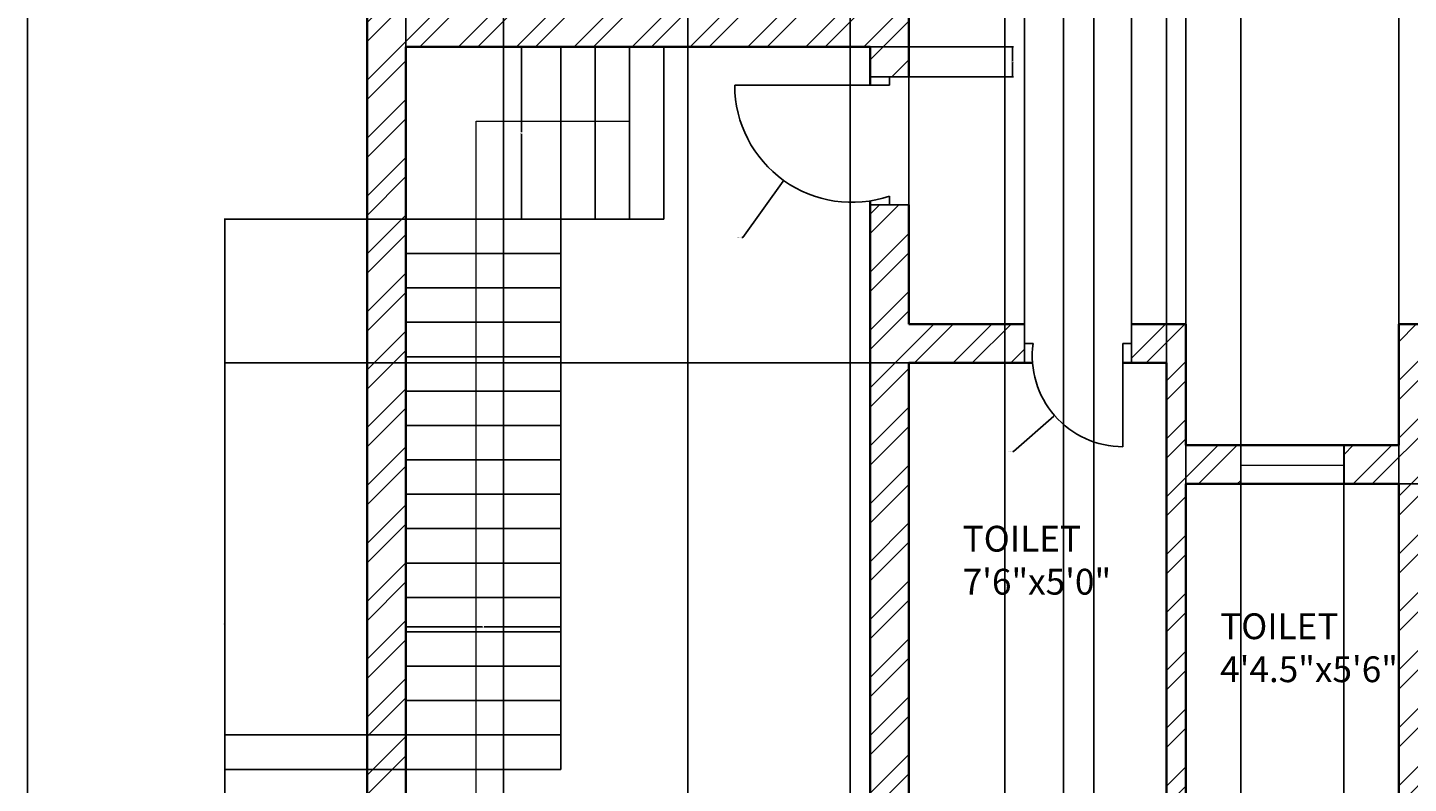
# Model space of a CAD drawing. Units: inches. Extents: x 1595 to 2135, y 460 to 2061.
# Tile 2 of 5: x 1595 to 1917, y 1470 to 1646. Entities that reach past the tile are written whole.
import ezdxf

# ---------------------------------------------------------------- set-up
doc = ezdxf.new("R2010")
doc.units = ezdxf.units.IN
for name, color, linetype, lineweight in [('A-ANNO-DIMS', 2, 'Continuous', 18), ('A-ANNO-SYMB', 7, 'Continuous', 18), ('A-ANNO-TTLB', 7, 'Continuous', 25), ('A-AREA-IDEN', 7, 'Continuous', 18), ('A-DOOR', 3, 'Continuous', 25), ('A-FLOR-STRS', 7, 'Continuous', 25), ('A-GLAZ', 4, 'Continuous', 18), ('A-WALL', 7, 'Continuous', 35)]:
    doc.layers.add(name, color=color, linetype=linetype, lineweight=lineweight)
doc.layers.add('A-WALL-PATT', color=143, linetype='Continuous', lineweight=13, true_color=0x7aafdf)
doc.styles.get("Standard").update_dxf_attribs({"font": 'arial.ttf'})
doc.dimstyles.get("Standard").update_dxf_attribs({"dimtxt": 0.18, "dimasz": 0.18, "dimexe": 0.18, "dimexo": 0.0625, "dimgap": 0.09, "dimtad": 0, "dimtih": 1, "dimtoh": 1, "dimdec": 4, "dimzin": 0, "dimdsep": 46, "dimtxsty": 'Standard', "dimcen": 0.09, "dimadec": 0, "dimazin": 0, "dimtfac": 1, "dimtdec": 4, "dimtofl": 0, "dimtmove": 0, "dimatfit": 3, "dimfxl": 1, "dimtolj": 1, "dimtzin": 0, "dimarcsym": 0})

# ---------------------------------------------------------------- blocks, each defined once
blk = doc.blocks.new('*D6')
at = {"layer": 'A-ANNO-DIMS', "color": 0, "lineweight": -2, "transparency": 16777216}
for p, q in [((1791.38, 1641.64), (1824.64, 1641.64)), ((1824.46, 1641.46), (1824.46, 1638.36)), ((1824.46, 1634.9), (1824.46, 1638)), ((1791.38, 1634.72), (1824.64, 1634.72))]:
    blk.add_line(p, q, dxfattribs=at)
at = {"layer": 'A-ANNO-DIMS', "color": 0, "transparency": 16777216}
for points in [[(1824.43, 1641.46), (1824.49, 1641.46), (1824.46, 1641.64)], [(1824.43, 1634.9), (1824.49, 1634.9), (1824.46, 1634.72)]]:
    blk.add_solid(points, dxfattribs=at)
at = {"layer": 'Defpoints', "color": 0, "transparency": 16777216}
for p in [(1791.31, 1641.64), (1791.31, 1634.72), (1824.46, 1634.72)]:
    blk.add_point(p, dxfattribs=at)
at = {"layer": 'A-ANNO-DIMS', "color": 0, "transparency": 16777216, "insert": (1824.46, 1638.18), "char_height": 0.18, "attachment_point": 5}
blk.add_mtext('\\A1;6.925', dxfattribs=at)
blk = doc.blocks.new('*D17')
at = {"layer": 'A-ANNO-DIMS', "color": 0, "lineweight": -2, "transparency": 16777216}
for p, q in [((1683.31, 1473.65), (1683.31, 1506.92)), ((1719.31, 1473.65), (1719.31, 1506.92)), ((1683.49, 1506.74), (1701.09, 1506.74)), ((1719.13, 1506.74), (1701.53, 1506.74))]:
    blk.add_line(p, q, dxfattribs=at)
at = {"layer": 'A-ANNO-DIMS', "color": 0, "transparency": 16777216}
for points in [[(1683.49, 1506.77), (1683.49, 1506.71), (1683.31, 1506.74)], [(1719.13, 1506.77), (1719.13, 1506.71), (1719.31, 1506.74)]]:
    blk.add_solid(points, dxfattribs=at)
at = {"layer": 'Defpoints', "color": 0, "transparency": 16777216}
for p in [(1719.31, 1506.74), (1683.31, 1473.59), (1719.31, 1473.59)]:
    blk.add_point(p, dxfattribs=at)
at = {"layer": 'A-ANNO-DIMS', "color": 0, "transparency": 16777216, "insert": (1701.31, 1506.74), "char_height": 0.18, "attachment_point": 5}
blk.add_mtext('\\A1;36', dxfattribs=at)
blk = doc.blocks.new('*D18')
at = {"layer": 'A-ANNO-DIMS', "color": 0, "lineweight": -2, "transparency": 16777216}
for p, q in [((1683.25, 1601.59), (1640.98, 1601.59)), ((1641.16, 1601.41), (1641.16, 1537.77)), ((1641.16, 1473.77), (1641.16, 1537.41)), ((1683.25, 1473.59), (1640.98, 1473.59))]:
    blk.add_line(p, q, dxfattribs=at)
at = {"layer": 'A-ANNO-DIMS', "color": 0, "transparency": 16777216}
for points in [[(1641.13, 1601.41), (1641.19, 1601.41), (1641.16, 1601.59)], [(1641.13, 1473.77), (1641.19, 1473.77), (1641.16, 1473.59)]]:
    blk.add_solid(points, dxfattribs=at)
at = {"layer": 'Defpoints', "color": 0, "transparency": 16777216}
for p in [(1641.16, 1601.59), (1683.31, 1601.59), (1683.31, 1473.59)]:
    blk.add_point(p, dxfattribs=at)
at = {"layer": 'A-ANNO-DIMS', "color": 0, "transparency": 16777216, "insert": (1641.16, 1537.59), "char_height": 0.18, "attachment_point": 5}
blk.add_mtext('\\A1;128', dxfattribs=at)
blk = doc.blocks.new('*D19')
at = {"layer": 'A-ANNO-DIMS', "color": 0, "lineweight": -2, "transparency": 16777216}
for p, q in [((1683.25, 1481.59), (1640.98, 1481.59)), ((1641.16, 1481.41), (1641.16, 1477.77)), ((1641.16, 1473.77), (1641.16, 1477.41)), ((1683.25, 1473.59), (1640.98, 1473.59))]:
    blk.add_line(p, q, dxfattribs=at)
at = {"layer": 'A-ANNO-DIMS', "color": 0, "transparency": 16777216}
for points in [[(1641.13, 1481.41), (1641.19, 1481.41), (1641.16, 1481.59)], [(1641.13, 1473.77), (1641.19, 1473.77), (1641.16, 1473.59)]]:
    blk.add_solid(points, dxfattribs=at)
at = {"layer": 'Defpoints', "color": 0, "transparency": 16777216}
for p in [(1641.16, 1481.59), (1683.31, 1481.59), (1683.31, 1473.59)]:
    blk.add_point(p, dxfattribs=at)
at = {"layer": 'A-ANNO-DIMS', "color": 0, "transparency": 16777216, "insert": (1641.16, 1477.59), "char_height": 0.18, "attachment_point": 5}
blk.add_mtext('\\A1;8', dxfattribs=at)
blk = doc.blocks.new('*D23')
at = {"layer": 'A-ANNO-DIMS', "color": 0, "lineweight": -2, "transparency": 16777216}
for p, q in [((1683.31, 1938.58), (1683.31, 1365.31)), ((1705.98, 1938.58), (1705.98, 1365.31)), ((1683.49, 1365.49), (1694.18, 1365.49)), ((1705.8, 1365.49), (1695.11, 1365.49))]:
    blk.add_line(p, q, dxfattribs=at)
at = {"layer": 'A-ANNO-DIMS', "color": 0, "transparency": 16777216}
for points in [[(1683.49, 1365.52), (1683.49, 1365.46), (1683.31, 1365.49)], [(1705.8, 1365.52), (1705.8, 1365.46), (1705.98, 1365.49)]]:
    blk.add_solid(points, dxfattribs=at)
at = {"layer": 'Defpoints', "color": 0, "transparency": 16777216}
for p in [(1683.31, 1938.64), (1705.98, 1938.64), (1705.98, 1365.49)]:
    blk.add_point(p, dxfattribs=at)
at = {"layer": 'A-ANNO-DIMS', "color": 0, "transparency": 16777216, "insert": (1694.64, 1365.49), "char_height": 0.18, "attachment_point": 5}
blk.add_mtext('\\A1;22.663', dxfattribs=at)
blk = doc.blocks.new('*D24')
at = {"layer": 'A-ANNO-DIMS', "color": 0, "lineweight": -2, "transparency": 16777216}
for p, q in [((1705.98, 1938.58), (1705.98, 1365.31)), ((1748.87, 1938.58), (1748.87, 1365.31)), ((1706.16, 1365.49), (1726.96, 1365.49)), ((1748.69, 1365.49), (1727.89, 1365.49))]:
    blk.add_line(p, q, dxfattribs=at)
at = {"layer": 'A-ANNO-DIMS', "color": 0, "transparency": 16777216}
for points in [[(1706.16, 1365.52), (1706.16, 1365.46), (1705.98, 1365.49)], [(1748.69, 1365.52), (1748.69, 1365.46), (1748.87, 1365.49)]]:
    blk.add_solid(points, dxfattribs=at)
at = {"layer": 'Defpoints', "color": 0, "transparency": 16777216}
for p in [(1705.98, 1938.64), (1748.87, 1938.64), (1748.87, 1365.49)]:
    blk.add_point(p, dxfattribs=at)
at = {"layer": 'A-ANNO-DIMS', "color": 0, "transparency": 16777216, "insert": (1727.42, 1365.49), "char_height": 0.18, "attachment_point": 5}
blk.add_mtext('\\A1;42.894', dxfattribs=at)
blk = doc.blocks.new('*D25')
at = {"layer": 'A-ANNO-DIMS', "color": 0, "lineweight": -2, "transparency": 16777216}
for p, q in [((1748.87, 1938.58), (1748.87, 1365.31)), ((1786.65, 1938.58), (1786.65, 1365.31)), ((1749.05, 1365.49), (1767.37, 1365.49)), ((1786.47, 1365.49), (1768.16, 1365.49))]:
    blk.add_line(p, q, dxfattribs=at)
at = {"layer": 'A-ANNO-DIMS', "color": 0, "transparency": 16777216}
for points in [[(1749.05, 1365.52), (1749.05, 1365.46), (1748.87, 1365.49)], [(1786.47, 1365.52), (1786.47, 1365.46), (1786.65, 1365.49)]]:
    blk.add_solid(points, dxfattribs=at)
at = {"layer": 'Defpoints', "color": 0, "transparency": 16777216}
for p in [(1748.87, 1938.64), (1786.65, 1938.64), (1786.65, 1365.49)]:
    blk.add_point(p, dxfattribs=at)
at = {"layer": 'A-ANNO-DIMS', "color": 0, "transparency": 16777216, "insert": (1767.76, 1365.49), "char_height": 0.18, "attachment_point": 5}
blk.add_mtext('\\A1;37.78', dxfattribs=at)
blk = doc.blocks.new('*D26')
at = {"layer": 'A-ANNO-DIMS', "color": 0, "lineweight": -2, "transparency": 16777216}
for p, q in [((1786.65, 1938.58), (1786.65, 1365.31)), ((1822.65, 1938.58), (1822.65, 1365.31)), ((1786.83, 1365.49), (1804.43, 1365.49)), ((1822.47, 1365.49), (1804.87, 1365.49))]:
    blk.add_line(p, q, dxfattribs=at)
at = {"layer": 'A-ANNO-DIMS', "color": 0, "transparency": 16777216}
for points in [[(1786.83, 1365.52), (1786.83, 1365.46), (1786.65, 1365.49)], [(1822.47, 1365.52), (1822.47, 1365.46), (1822.65, 1365.49)]]:
    blk.add_solid(points, dxfattribs=at)
at = {"layer": 'Defpoints', "color": 0, "transparency": 16777216}
for p in [(1786.65, 1938.64), (1822.65, 1938.64), (1822.65, 1365.49)]:
    blk.add_point(p, dxfattribs=at)
at = {"layer": 'A-ANNO-DIMS', "color": 0, "transparency": 16777216, "insert": (1804.65, 1365.49), "char_height": 0.18, "attachment_point": 5}
blk.add_mtext('\\A1;36', dxfattribs=at)
blk = doc.blocks.new('*D30')
at = {"layer": 'A-ANNO-DIMS', "color": 0, "lineweight": -2, "transparency": 16777216}
for p, q in [((1836.31, 1938.58), (1836.31, 1365.31)), ((1843.37, 1938.58), (1843.37, 1365.31)), ((1836.49, 1365.49), (1839.45, 1365.49)), ((1843.19, 1365.49), (1840.23, 1365.49))]:
    blk.add_line(p, q, dxfattribs=at)
at = {"layer": 'A-ANNO-DIMS', "color": 0, "transparency": 16777216}
for points in [[(1836.49, 1365.52), (1836.49, 1365.46), (1836.31, 1365.49)], [(1843.19, 1365.52), (1843.19, 1365.46), (1843.37, 1365.49)]]:
    blk.add_solid(points, dxfattribs=at)
at = {"layer": 'Defpoints', "color": 0, "transparency": 16777216}
for p in [(1836.31, 1938.64), (1843.37, 1938.64), (1843.37, 1365.49)]:
    blk.add_point(p, dxfattribs=at)
at = {"layer": 'A-ANNO-DIMS', "color": 0, "transparency": 16777216, "insert": (1839.84, 1365.49), "char_height": 0.18, "attachment_point": 5}
blk.add_mtext('\\A1;7.054', dxfattribs=at)
blk = doc.blocks.new('*D33')
at = {"layer": 'A-ANNO-DIMS', "color": 0, "lineweight": -2, "transparency": 16777216}
for p, q in [((1800.25, 1568.14), (1640.98, 1568.14)), ((1641.16, 1567.96), (1641.16, 1507.57)), ((1641.16, 1446.82), (1641.16, 1507.21)), ((1800.25, 1446.64), (1640.98, 1446.64))]:
    blk.add_line(p, q, dxfattribs=at)
at = {"layer": 'A-ANNO-DIMS', "color": 0, "transparency": 16777216}
for points in [[(1641.13, 1567.96), (1641.19, 1567.96), (1641.16, 1568.14)], [(1641.13, 1446.82), (1641.19, 1446.82), (1641.16, 1446.64)]]:
    blk.add_solid(points, dxfattribs=at)
at = {"layer": 'Defpoints', "color": 0, "transparency": 16777216}
for p in [(1641.16, 1568.14), (1800.31, 1568.14), (1800.31, 1446.64)]:
    blk.add_point(p, dxfattribs=at)
at = {"layer": 'A-ANNO-DIMS', "color": 0, "transparency": 16777216, "insert": (1641.16, 1507.39), "char_height": 0.18, "attachment_point": 5}
blk.add_mtext('\\A1;121.5', dxfattribs=at)
blk = doc.blocks.new('*D34')
at = {"layer": 'A-ANNO-DIMS', "color": 0, "lineweight": -2, "transparency": 16777216}
for p, q in [((1914.38, 1539.98), (2109.64, 1539.98)), ((2109.46, 1539.8), (2109.46, 1493.49)), ((2109.46, 1446.82), (2109.46, 1493.13)), ((1914.38, 1446.64), (2109.64, 1446.64))]:
    blk.add_line(p, q, dxfattribs=at)
at = {"layer": 'A-ANNO-DIMS', "color": 0, "transparency": 16777216}
for points in [[(2109.43, 1539.8), (2109.49, 1539.8), (2109.46, 1539.98)], [(2109.43, 1446.82), (2109.49, 1446.82), (2109.46, 1446.64)]]:
    blk.add_solid(points, dxfattribs=at)
at = {"layer": 'Defpoints', "color": 0, "transparency": 16777216}
for p in [(1914.31, 1539.98), (2109.46, 1539.98), (1914.31, 1446.64)]:
    blk.add_point(p, dxfattribs=at)
at = {"layer": 'A-ANNO-DIMS', "color": 0, "transparency": 16777216, "insert": (2109.46, 1493.31), "char_height": 0.18, "attachment_point": 5}
blk.add_mtext('\\A1;93.33', dxfattribs=at)
blk = doc.blocks.new('*D35')
at = {"layer": 'A-ANNO-DIMS', "color": 0, "lineweight": -2, "transparency": 16777216}
for p, q in [((1864.81, 1540.04), (1864.81, 2049.97)), ((1914.31, 1540.04), (1914.31, 2049.97)), ((1864.99, 2049.79), (1889.23, 2049.79)), ((1914.13, 2049.79), (1889.89, 2049.79))]:
    blk.add_line(p, q, dxfattribs=at)
at = {"layer": 'A-ANNO-DIMS', "color": 0, "transparency": 16777216}
for points in [[(1864.99, 2049.82), (1864.99, 2049.76), (1864.81, 2049.79)], [(1914.13, 2049.82), (1914.13, 2049.76), (1914.31, 2049.79)]]:
    blk.add_solid(points, dxfattribs=at)
at = {"layer": 'Defpoints', "color": 0, "transparency": 16777216}
for p in [(1914.31, 2049.79), (1864.81, 1539.98), (1914.31, 1539.98)]:
    blk.add_point(p, dxfattribs=at)
at = {"layer": 'A-ANNO-DIMS', "color": 0, "transparency": 16777216, "insert": (1889.56, 2049.79), "char_height": 0.18, "attachment_point": 5}
blk.add_mtext('\\A1;49.5', dxfattribs=at)
blk = doc.blocks.new('*D36')
at = {"layer": 'A-ANNO-DIMS', "color": 0, "lineweight": -2, "transparency": 16777216}
for p, q in [((1860.31, 1568.2), (1860.31, 2049.97)), ((1864.81, 1577.2), (1864.81, 2049.97)), ((1860.49, 2049.79), (1862.3, 2049.79)), ((1864.63, 2049.79), (1862.82, 2049.79))]:
    blk.add_line(p, q, dxfattribs=at)
at = {"layer": 'A-ANNO-DIMS', "color": 0, "transparency": 16777216}
for points in [[(1860.49, 2049.82), (1860.49, 2049.76), (1860.31, 2049.79)], [(1864.63, 2049.82), (1864.63, 2049.76), (1864.81, 2049.79)]]:
    blk.add_solid(points, dxfattribs=at)
at = {"layer": 'Defpoints', "color": 0, "transparency": 16777216}
for p in [(1864.81, 2049.79), (1864.81, 1577.14), (1860.31, 1568.14)]:
    blk.add_point(p, dxfattribs=at)
at = {"layer": 'A-ANNO-DIMS', "color": 0, "transparency": 16777216, "insert": (1862.56, 2049.79), "char_height": 0.18, "attachment_point": 5}
blk.add_mtext('\\A1;4.5', dxfattribs=at)
blk = doc.blocks.new('*D37')
at = {"layer": 'A-ANNO-DIMS', "color": 0, "lineweight": -2, "transparency": 16777216}
for p, q in [((1800.31, 1577.2), (1800.31, 2049.97)), ((1827.24, 1577.2), (1827.24, 2049.97)), ((1800.49, 2049.79), (1813.31, 2049.79)), ((1827.06, 2049.79), (1814.24, 2049.79))]:
    blk.add_line(p, q, dxfattribs=at)
at = {"layer": 'A-ANNO-DIMS', "color": 0, "transparency": 16777216}
for points in [[(1800.49, 2049.82), (1800.49, 2049.76), (1800.31, 2049.79)], [(1827.06, 2049.82), (1827.06, 2049.76), (1827.24, 2049.79)]]:
    blk.add_solid(points, dxfattribs=at)
at = {"layer": 'Defpoints', "color": 0, "transparency": 16777216}
for p in [(1827.24, 2049.79), (1800.31, 1577.14), (1827.24, 1577.14)]:
    blk.add_point(p, dxfattribs=at)
at = {"layer": 'A-ANNO-DIMS', "color": 0, "transparency": 16777216, "insert": (1813.78, 2049.79), "char_height": 0.18, "attachment_point": 5}
blk.add_mtext('\\A1;26.927', dxfattribs=at)
blk = doc.blocks.new('*D38')
at = {"layer": 'A-ANNO-DIMS', "color": 0, "lineweight": -2, "transparency": 16777216}
for p, q in [((1827.24, 1577.2), (1827.24, 2049.97)), ((1852.14, 1577.2), (1852.14, 2049.97)), ((1827.42, 2049.79), (1839.23, 2049.79)), ((1851.96, 2049.79), (1840.16, 2049.79))]:
    blk.add_line(p, q, dxfattribs=at)
at = {"layer": 'A-ANNO-DIMS', "color": 0, "transparency": 16777216}
for points in [[(1827.42, 2049.82), (1827.42, 2049.76), (1827.24, 2049.79)], [(1851.96, 2049.82), (1851.96, 2049.76), (1852.14, 2049.79)]]:
    blk.add_solid(points, dxfattribs=at)
at = {"layer": 'Defpoints', "color": 0, "transparency": 16777216}
for p in [(1852.14, 2049.79), (1827.24, 1577.14), (1852.14, 1577.14)]:
    blk.add_point(p, dxfattribs=at)
at = {"layer": 'A-ANNO-DIMS', "color": 0, "transparency": 16777216, "insert": (1839.69, 2049.79), "char_height": 0.18, "attachment_point": 5}
blk.add_mtext('\\A1;24.904', dxfattribs=at)
blk = doc.blocks.new('*D43')
at = {"layer": 'A-ANNO-DIMS', "color": 0, "lineweight": -2, "transparency": 16777216}
for p, q in [((1877.58, 1548.91), (1877.58, 1365.31)), ((1901.58, 1548.91), (1901.58, 1365.31)), ((1877.76, 1365.49), (1889.36, 1365.49)), ((1901.4, 1365.49), (1889.8, 1365.49))]:
    blk.add_line(p, q, dxfattribs=at)
at = {"layer": 'A-ANNO-DIMS', "color": 0, "transparency": 16777216}
for points in [[(1877.76, 1365.52), (1877.76, 1365.46), (1877.58, 1365.49)], [(1901.4, 1365.52), (1901.4, 1365.46), (1901.58, 1365.49)]]:
    blk.add_solid(points, dxfattribs=at)
at = {"layer": 'Defpoints', "color": 0, "transparency": 16777216}
for p in [(1877.58, 1548.98), (1901.58, 1548.98), (1901.58, 1365.49)]:
    blk.add_point(p, dxfattribs=at)
at = {"layer": 'A-ANNO-DIMS', "color": 0, "transparency": 16777216, "insert": (1889.58, 1365.49), "char_height": 0.18, "attachment_point": 5}
blk.add_mtext('\\A1;24', dxfattribs=at)
blk = doc.blocks.new('*D44')
at = {"layer": 'A-ANNO-DIMS', "color": 0, "lineweight": -2, "transparency": 16777216}
for p, q in [((1864.81, 1549.04), (1864.81, 2049.97)), ((1877.58, 1549.04), (1877.58, 2049.97)), ((1864.99, 2049.79), (1870.74, 2049.79)), ((1877.4, 2049.79), (1871.65, 2049.79))]:
    blk.add_line(p, q, dxfattribs=at)
at = {"layer": 'A-ANNO-DIMS', "color": 0, "transparency": 16777216}
for points in [[(1864.99, 2049.82), (1864.99, 2049.76), (1864.81, 2049.79)], [(1877.4, 2049.82), (1877.4, 2049.76), (1877.58, 2049.79)]]:
    blk.add_solid(points, dxfattribs=at)
at = {"layer": 'Defpoints', "color": 0, "transparency": 16777216}
for p in [(1877.58, 2049.79), (1864.81, 1548.98), (1877.58, 1548.98)]:
    blk.add_point(p, dxfattribs=at)
at = {"layer": 'A-ANNO-DIMS', "color": 0, "transparency": 16777216, "insert": (1871.2, 2049.79), "char_height": 0.18, "attachment_point": 5}
blk.add_mtext('\\A1;12.769', dxfattribs=at)
blk = doc.blocks.new('*D47')
at = {"layer": 'A-ANNO-DIMS', "color": 0, "lineweight": -2, "transparency": 16777216}
for p, q in [((1683.25, 1473.59), (1640.98, 1473.59)), ((1641.16, 1473.41), (1641.16, 1440.8)), ((1641.16, 1407.82), (1641.16, 1440.44)), ((1683.25, 1407.64), (1640.98, 1407.64))]:
    blk.add_line(p, q, dxfattribs=at)
at = {"layer": 'A-ANNO-DIMS', "color": 0, "transparency": 16777216}
for points in [[(1641.13, 1473.41), (1641.19, 1473.41), (1641.16, 1473.59)], [(1641.13, 1407.82), (1641.19, 1407.82), (1641.16, 1407.64)]]:
    blk.add_solid(points, dxfattribs=at)
at = {"layer": 'Defpoints', "color": 0, "transparency": 16777216}
for p in [(1641.16, 1473.59), (1683.31, 1473.59), (1683.31, 1407.64)]:
    blk.add_point(p, dxfattribs=at)
at = {"layer": 'A-ANNO-DIMS', "color": 0, "transparency": 16777216, "insert": (1641.16, 1440.62), "char_height": 0.18, "attachment_point": 5}
blk.add_mtext('\\A1;65.95', dxfattribs=at)
blk = doc.blocks.new('*D48')
at = {"layer": 'A-ANNO-DIMS', "color": 0, "lineweight": -2, "transparency": 16777216}
for p, q in [((1743.25, 1641.64), (1709.98, 1641.64)), ((1710.16, 1641.46), (1710.16, 1621.8)), ((1710.16, 1601.77), (1710.16, 1621.44)), ((1743.25, 1601.59), (1709.98, 1601.59))]:
    blk.add_line(p, q, dxfattribs=at)
at = {"layer": 'A-ANNO-DIMS', "color": 0, "transparency": 16777216}
for points in [[(1710.13, 1641.46), (1710.19, 1641.46), (1710.16, 1641.64)], [(1710.13, 1601.77), (1710.19, 1601.77), (1710.16, 1601.59)]]:
    blk.add_solid(points, dxfattribs=at)
at = {"layer": 'Defpoints', "color": 0, "transparency": 16777216}
for p in [(1710.16, 1641.64), (1743.31, 1641.64), (1743.31, 1601.59)]:
    blk.add_point(p, dxfattribs=at)
at = {"layer": 'A-ANNO-DIMS', "color": 0, "transparency": 16777216, "insert": (1710.16, 1621.62), "char_height": 0.18, "attachment_point": 5}
blk.add_mtext('\\A1;40.05', dxfattribs=at)
blk = doc.blocks.new('*D60')
at = {"layer": 'A-ANNO-DIMS', "color": 0, "lineweight": -2, "transparency": 16777216}
for p, q in [((1786.95, 1632.72), (1787.13, 1632.72)), ((1787.04, 1632.63), (1787.04, 1632.81)), ((1761.68, 1597.3), (1771.09, 1610.43)), ((1761.5, 1597.3), (1761.68, 1597.3))]:
    blk.add_line(p, q, dxfattribs=at)
at = {"layer": 'A-ANNO-DIMS', "color": 0, "transparency": 16777216}
blk.add_solid([(1771.06, 1610.45), (1771.11, 1610.42), (1771.19, 1610.58)], dxfattribs=at)
at = {"layer": 'Defpoints', "color": 0, "transparency": 16777216}
for p in [(1787.04, 1632.72), (1771.19, 1610.58)]:
    blk.add_point(p, dxfattribs=at)
at = {"layer": 'A-ANNO-DIMS', "color": 0, "transparency": 16777216, "insert": (1760.95, 1597.3), "char_height": 0.18, "attachment_point": 5}
blk.add_mtext('\\A1;R27.223', dxfattribs=at)
blk = doc.blocks.new('*D63')
at = {"layer": 'A-ANNO-DIMS', "color": 0, "lineweight": -2, "transparency": 16777216}
for p, q in [((1850.05, 1569.75), (1850.23, 1569.75)), ((1850.14, 1569.66), (1850.14, 1569.84)), ((1824.68, 1547.57), (1834.09, 1555.77)), ((1824.5, 1547.57), (1824.68, 1547.57))]:
    blk.add_line(p, q, dxfattribs=at)
at = {"layer": 'A-ANNO-DIMS', "color": 0, "transparency": 16777216}
blk.add_solid([(1834.07, 1555.79), (1834.11, 1555.74), (1834.23, 1555.89)], dxfattribs=at)
at = {"layer": 'Defpoints', "color": 0, "transparency": 16777216}
for p in [(1850.14, 1569.75), (1834.23, 1555.89)]:
    blk.add_point(p, dxfattribs=at)
at = {"layer": 'A-ANNO-DIMS', "color": 0, "transparency": 16777216, "insert": (1823.95, 1547.57), "char_height": 0.18, "attachment_point": 5}
blk.add_mtext('\\A1;R21.104', dxfattribs=at)

msp = doc.modelspace()

# ---------------------------------------------------------------- hatches: boundary and pattern name
at = {"layer": 'A-WALL-PATT'}
h = msp.add_hatch(dxfattribs=at)
h.set_pattern_fill('ANSI32', color=256)
h.paths.add_polyline_path([(2076.313, 2016.6421), (1674.313, 2016.6421), (1674.313, 1905.0731), (1683.313, 1905.0731), (1683.313, 1938.6421), (1705.9756, 1938.6421), (1705.9756, 1947.6421), (1683.313, 1947.6421), (1683.313, 2007.6421), (2067.313, 2007.6421), (2067.313, 1947.6421), (2046.0304, 1947.6421), (2046.0304, 1938.6421), (2067.313, 1938.6421), (2067.313, 1906.0373), (2076.313, 1906.0373), (2076.313, 1947.6421)])
h.paths.add_polyline_path([(1786.653, 1947.6421), (1748.8699, 1947.6421), (1748.8699, 1938.6421), (1786.653, 1938.6421), (1786.653, 1943.1421)], flags=17)
h.paths.add_polyline_path([(1843.367, 1943.1421), (1843.367, 1947.6421), (1822.653, 1947.6421), (1822.653, 1938.6421), (1827.313, 1938.6421), (1827.313, 1821.1082), (1836.313, 1821.1082), (1836.313, 1938.6421), (1843.367, 1938.6421)])
h.paths.add_polyline_path([(1928.933, 1943.1421), (1928.933, 1947.6421), (1875.313, 1947.6421), (1875.313, 1938.6421), (1914.313, 1938.6421), (1914.313, 1820.8892), (1923.313, 1820.8892), (1923.313, 1938.6421), (1928.933, 1938.6421)])
h.paths.add_polyline_path([(1997.1133, 1947.6421), (1964.933, 1947.6421), (1964.933, 1938.6421), (1997.1133, 1938.6421)], flags=17)
h.paths.add_polyline_path([(1974.313, 2007.6421), (1969.813, 2007.6421), (1969.813, 1947.6421), (1974.313, 1947.6421)], flags=17)
h.paths.add_polyline_path([(1780.813, 2007.6421), (1776.313, 2007.6421), (1776.313, 1947.6421), (1780.813, 1947.6421)], flags=17)
h.paths.add_polyline_path([(1683.313, 1845.0731), (1674.313, 1845.0731), (1674.313, 1734.209), (1683.313, 1734.209), (1683.313, 1773.6421), (1795.813, 1773.6421), (1836.313, 1773.6421), (1836.313, 1788.3627), (1831.813, 1788.3627), (1827.313, 1788.3627), (1827.313, 1782.6421), (1683.313, 1782.6421)])
h.paths.add_polyline_path([(2076.313, 1846.0373), (2067.313, 1846.0373), (2067.313, 1782.6421), (1923.313, 1782.6421), (1923.313, 1788.8802), (1918.813, 1788.8802), (1914.313, 1788.8802), (1914.313, 1773.6421), (2067.313, 1773.6421), (2067.313, 1710.6421), (2076.313, 1710.6421)])
h.paths.add_polyline_path([(1844.0531, 1859.9747), (1909.4596, 1859.9747), (1909.4596, 1882.3635), (1844.0531, 1882.3635)], flags=9)
h.paths.add_polyline_path([(1721.6058, 1827.3507), (1768.2143, 1827.3507), (1768.2143, 1849.7395), (1721.6058, 1849.7395)], flags=9)
h.paths.add_polyline_path([(1786.8661, 1359.2872), (1978.2276, 1359.2872), (1978.2276, 1384.0157), (1786.8661, 1384.0157)], flags=9)
h.paths.add_polyline_path([(1795.7228, 1412.0413), (1871.5904, 1412.0413), (1871.5904, 1424.4055), (1795.7228, 1424.4055)], flags=9)
h.paths.add_polyline_path([(1954.3634, 1526.3976), (2013.549, 1526.3976), (2013.549, 1548.7864), (1954.3634, 1548.7864)], flags=9)
h.paths.add_polyline_path([(1871.0596, 1490.4707), (1913.1292, 1490.4707), (1913.1292, 1512.8595), (1871.0596, 1512.8595)], flags=9)
h.paths.add_polyline_path([(1810.9452, 1510.8402), (1845.9343, 1510.8402), (1845.9343, 1533.229), (1810.9452, 1533.229)], flags=9)
h.paths.add_polyline_path([(1720.9117, 1692.9695), (1767.819, 1692.9695), (1767.819, 1715.3583), (1720.9117, 1715.3583)], flags=9)
h.paths.add_polyline_path([(1853.0254, 1698.4614), (1904.6966, 1698.4614), (1904.6966, 1720.8503), (1853.0254, 1720.8503)], flags=9)
h.paths.add_polyline_path([(1970.399, 1827.3507), (2017.0075, 1827.3507), (2017.0075, 1849.7395), (1970.399, 1849.7395)], flags=9)
h.paths.add_polyline_path([(1994.3418, 1955.5613), (2029.5928, 1955.5613), (2029.5928, 1977.9501), (1994.3418, 1977.9501)], flags=25)
h.paths.add_polyline_path([(1828.8665, 1964.6116), (1868.5173, 1964.6116), (1868.5173, 1987.0004), (1828.8665, 1987.0004)], flags=25)
h.paths.add_polyline_path([(1698.1483, 1960.8371), (1733.3994, 1960.8371), (1733.3994, 1983.2259), (1698.1483, 1983.2259)], flags=25)
h = msp.add_hatch(dxfattribs=at)
h.set_pattern_fill('ANSI32', color=256)
h.paths.add_polyline_path([(1683.313, 1641.6421), (1791.313, 1641.6421), (1791.313, 1634.7169), (1800.313, 1634.7169), (1800.313, 1650.6421), (1800.313, 1673.3054), (1795.813, 1673.3054), (1795.813, 1650.6421), (1683.313, 1650.6421), (1683.313, 1698.209), (1678.813, 1698.209), (1674.313, 1698.209), (1674.313, 1398.6421), (1688.853, 1398.6421), (1688.853, 1403.1421), (1688.853, 1407.6421), (1683.313, 1407.6421)])
h.paths.add_polyline_path([(1800.313, 1568.1421), (1827.2399, 1568.1421), (1827.2399, 1572.6421), (1827.2399, 1577.1421), (1800.313, 1577.1421), (1800.313, 1604.9472), (1795.813, 1604.9472), (1791.313, 1604.9472), (1791.313, 1437.6421), (1800.313, 1437.6421), (1815.6708, 1437.6421), (1815.6708, 1442.1421), (1815.6708, 1446.6421), (1800.313, 1446.6421)])
h.paths.add_polyline_path([(1877.5816, 1545.4284), (1877.5816, 1548.9761), (1864.813, 1548.9761), (1864.813, 1577.1421), (1852.144, 1577.1421), (1852.144, 1568.1421), (1860.313, 1568.1421), (1860.313, 1446.6421), (1839.6708, 1446.6421), (1839.6708, 1437.6421), (1869.0647, 1437.6421), (1869.0647, 1442.1421), (1869.0647, 1446.6421), (1864.813, 1446.6421), (1864.813, 1539.9761), (1877.5816, 1539.9761), (1877.5816, 1541.8808)])
h.paths.add_polyline_path([(1923.313, 1568.1421), (1936.607, 1568.1421), (1936.607, 1577.1421), (1914.313, 1577.1421), (1914.313, 1548.9761), (1901.5816, 1548.9761), (1901.5816, 1539.9761), (1914.313, 1539.9761), (1914.313, 1446.6421), (1891.5684, 1446.6421), (1891.5684, 1437.6421), (1914.313, 1437.6421), (1923.313, 1437.6421)])
h.paths.add_polyline_path([(2067.313, 1577.1421), (2003.1294, 1577.1421), (2003.1294, 1568.1421), (2067.313, 1568.1421)])
h.paths.add_polyline_path([(2076.313, 1650.6421), (2067.313, 1650.6421), (2067.313, 1504.2035), (2076.313, 1504.2035)])
h.paths.add_polyline_path([(2076.313, 1444.2035), (2071.813, 1444.2035), (2067.313, 1444.2035), (2067.313, 1407.6421), (1923.313, 1407.6421), (1918.813, 1407.6421), (1914.313, 1407.6421), (1737.2767, 1407.6421), (1737.2767, 1398.6421), (2076.313, 1398.6421)])

# ---------------------------------------------------------------- linework, layer by layer
at = {"layer": 'A-ANNO-SYMB'}
for p, q in [((1699.6809, 1459.3163), (1699.6809, 1624.3644)), ((1699.6809, 1624.3644), (1735.313, 1624.3644))]:
    msp.add_line(p, q, dxfattribs=at)
at = {"layer": 'A-ANNO-TTLB'}
msp.add_lwpolyline([(1595.2754, 2061.0707), (2134.6206, 2061.0707), (2134.6206, 1319.9937), (1595.2754, 1319.9937)], close=True, dxfattribs=at)
at = {"layer": 'A-DOOR'}
for p, q in [((1795.813, 1632.7169), (1759.813, 1632.7169)), ((1791.313, 1634.7169), (1800.313, 1634.7169)), ((1800.313, 1634.7169), (1795.813, 1634.7169)), ((1795.813, 1634.7169), (1795.813, 1632.7169)), ((1795.813, 1604.9472), (1795.813, 1606.9472)), ((1791.313, 1604.9472), (1800.313, 1604.9472)), ((1800.313, 1604.9472), (1795.813, 1604.9472)), ((1827.2399, 1577.1421), (1827.2399, 1568.1421)), ((1852.144, 1577.1421), (1852.144, 1568.1421)), ((1827.2399, 1568.1421), (1827.2399, 1572.6421)), ((1827.2399, 1572.6421), (1829.2399, 1572.6421)), ((1852.144, 1572.6421), (1850.144, 1572.6421)), ((1850.144, 1572.6421), (1850.144, 1548.6421)), ((1852.144, 1568.1421), (1852.144, 1572.6421))]:
    msp.add_line(p, q, dxfattribs=at)
for centre, radius, start, end in [((1787.0364, 1632.7169), 27.2233, 180, 288.807867), ((1850.144, 1569.7459), 21.1039, 172.112242, 270)]:
    msp.add_arc(centre, radius, start, end, dxfattribs=at)
at = {"layer": 'A-FLOR-STRS'}
for p, q in [((1719.313, 1473.5918), (1719.313, 1641.6421)), ((1719.313, 1641.6421), (1719.313, 1605.6421)), ((1727.313, 1609.5918), (1727.313, 1641.6421)), ((1727.313, 1641.6421), (1735.313, 1641.6421)), ((1735.313, 1641.6421), (1735.313, 1601.5918)), ((1743.313, 1601.5918), (1743.313, 1641.6421)), ((1727.313, 1601.5918), (1727.313, 1609.5918)), ((1683.313, 1601.5918), (1719.313, 1601.5918)), ((1719.313, 1601.5918), (1727.313, 1601.5918)), ((1735.313, 1601.5918), (1727.313, 1601.5918)), ((1735.313, 1601.5918), (1743.313, 1601.5918)), ((1735.313, 1601.5918), (1735.313, 1601.5918)), ((1683.313, 1593.5918), (1719.313, 1593.5918)), ((1683.313, 1585.5918), (1719.313, 1585.5918)), ((1683.313, 1577.5918), (1719.313, 1577.5918)), ((1683.313, 1569.5918), (1719.313, 1569.5918)), ((1683.313, 1561.5918), (1719.313, 1561.5918)), ((1683.313, 1553.5918), (1719.313, 1553.5918)), ((1683.313, 1545.5918), (1719.313, 1545.5918)), ((1683.313, 1537.5918), (1719.313, 1537.5918)), ((1683.313, 1529.5918), (1719.313, 1529.5918)), ((1683.313, 1521.5918), (1719.313, 1521.5918)), ((1683.313, 1513.5918), (1719.313, 1513.5918)), ((1683.313, 1505.5918), (1719.313, 1505.5918)), ((1683.313, 1497.5918), (1719.313, 1497.5918)), ((1683.313, 1489.5918), (1719.313, 1489.5918)), ((1683.313, 1481.5918), (1719.313, 1481.5918)), ((1683.313, 1473.5918), (1719.313, 1473.5918)), ((1719.313, 1473.5918), (1683.313, 1473.5918)), ((1791.313, 1473.5918), (1791.313, 1473.5918))]:
    msp.add_line(p, q, dxfattribs=at)
at = {"layer": 'A-GLAZ'}
for p, q in [((1877.5816, 1548.9761), (1877.5816, 1541.8808)), ((1901.5816, 1545.4284), (1901.5816, 1548.9761)), ((1901.5816, 1548.9761), (1901.5816, 1539.9761)), ((1877.5816, 1541.8808), (1877.5816, 1545.4284)), ((1877.5816, 1545.4284), (1877.5816, 1545.4284)), ((1877.5816, 1544.3563), (1901.5816, 1544.3563)), ((1877.5816, 1541.8808), (1877.5816, 1539.9761))]:
    msp.add_line(p, q, dxfattribs=at)
at = {"layer": 'A-WALL'}
for p, q in [((1674.313, 2016.6421), (1674.313, 1398.6421)), ((1800.313, 1650.6421), (1800.313, 1634.7169)), ((1683.313, 1641.6421), (1791.313, 1641.6421)), ((1683.313, 1641.6421), (1683.313, 1407.6421)), ((1791.313, 1632.7169), (1791.313, 1641.6421)), ((1791.313, 1437.6421), (1791.313, 1605.8316)), ((1800.313, 1604.9472), (1800.313, 1577.1421)), ((1800.313, 1577.1421), (1827.2399, 1577.1421)), ((1852.144, 1577.1421), (1864.813, 1577.1421)), ((1864.813, 1568.1421), (1864.813, 1577.1421)), ((1864.813, 1577.1421), (1864.813, 1548.9761)), ((1914.313, 1577.1421), (1914.313, 1548.9761)), ((1914.313, 1577.1421), (1936.607, 1577.1421)), ((1800.313, 1568.1421), (1829.1012, 1568.1421)), ((1800.313, 1568.1421), (1800.313, 1446.6421)), ((1850.144, 1568.1421), (1860.313, 1568.1421)), ((1860.313, 1568.1421), (1860.313, 1446.6421)), ((1864.813, 1548.9761), (1864.813, 1568.1421)), ((1914.313, 1548.9761), (1864.813, 1548.9761)), ((1864.813, 1446.6421), (1864.813, 1539.9761)), ((1864.813, 1539.9761), (1914.313, 1539.9761)), ((1914.313, 1539.9761), (1914.313, 1446.6421))]:
    msp.add_line(p, q, dxfattribs=at)

# ---------------------------------------------------------------- texts
at = {"layer": 'A-AREA-IDEN', "char_height": 6, "attachment_point": 1}
for s, width, insert in [('TOILET\\P7\'6"x5\'0"', 93.368305, (1812.8422, 1530.2474)), ('TOILET\\P4\'4.5"x5\'6"', 108.878995, (1872.756, 1509.8779))]:
    msp.add_mtext_dynamic_manual_height_columns(s, width=width, gutter_width=12.5, heights=[0], dxfattribs=dict(at, insert=insert))

# ---------------------------------------------------------------- dimensions: what is measured, and where the dimension line sits
at = {"layer": 'A-ANNO-DIMS'}
for base, p1, p2, override, picture, middle in [((1827.2399, 2049.7921), (1800.313, 1577.1421), (1827.2399, 1577.1421), {"dimdec": 3, "dimlfac": 1, "dimrnd": 0, "dimzin": 0, "dimdsep": 46, "dimlunit": 2}, '*D37', (1813.7764, 2049.7921)), ((1852.144, 2049.7921), (1827.2399, 1577.1421), (1852.144, 1577.1421), {"dimdec": 3, "dimlfac": 1, "dimrnd": 0, "dimzin": 0, "dimdsep": 46, "dimlunit": 2}, '*D38', (1839.6919, 2049.7921)), ((1864.813, 2049.7921), (1860.313, 1568.1421), (1864.813, 1577.1421), {"dimdec": 1, "dimlfac": 1, "dimrnd": 0, "dimzin": 0, "dimdsep": 46, "dimlunit": 2}, '*D36', (1862.563, 2049.7921)), ((1914.313, 2049.7921), (1864.813, 1539.9761), (1914.313, 1539.9761), {"dimdec": 1, "dimlfac": 1, "dimrnd": 0, "dimzin": 0, "dimdsep": 46, "dimlunit": 2}, '*D35', (1889.563, 2049.7921)), ((1877.5816, 2049.7921), (1864.813, 1548.9761), (1877.5816, 1548.9761), {"dimdec": 3, "dimlfac": 1, "dimrnd": 0, "dimzin": 0, "dimdsep": 46, "dimlunit": 2}, '*D44', (1871.1973, 2049.7921)), ((1705.9756, 1365.4921), (1683.313, 1938.6421), (1705.9756, 1938.6421), {"dimdec": 3, "dimlfac": 1, "dimrnd": 0, "dimzin": 0, "dimdsep": 46, "dimlunit": 2}, '*D23', (1694.6443, 1365.4921)), ((1748.8699, 1365.4921), (1705.9756, 1938.6421), (1748.8699, 1938.6421), {"dimdec": 3, "dimlfac": 1, "dimrnd": 0, "dimzin": 0, "dimdsep": 46, "dimlunit": 2}, '*D24', (1727.4227, 1365.4921)), ((1786.653, 1365.4921), (1748.8699, 1938.6421), (1786.653, 1938.6421), {"dimdec": 2, "dimlfac": 1, "dimrnd": 0, "dimzin": 0, "dimdsep": 46, "dimlunit": 2}, '*D25', (1767.7614, 1365.4921)), ((1822.653, 1365.4921), (1786.653, 1938.6421), (1822.653, 1938.6421), {"dimdec": 0, "dimlfac": 1, "dimrnd": 0, "dimzin": 0, "dimdsep": 46, "dimlunit": 2}, '*D26', (1804.653, 1365.4921)), ((1843.367, 1365.4921), (1836.313, 1938.6421), (1843.367, 1938.6421), {"dimdec": 3, "dimlfac": 1, "dimrnd": 0, "dimzin": 0, "dimdsep": 46, "dimlunit": 2}, '*D30', (1839.84, 1365.4921)), ((1901.5816, 1365.4921), (1877.5816, 1548.9761), (1901.5816, 1548.9761), {"dimdec": 0, "dimlfac": 1, "dimrnd": 0, "dimzin": 0, "dimdsep": 46, "dimlunit": 2}, '*D43', (1889.5816, 1365.4921)), ((1719.313, 1506.7418), (1683.313, 1473.5918), (1719.313, 1473.5918), {"dimdec": 0, "dimlfac": 1, "dimrnd": 0, "dimzin": 0, "dimdsep": 46, "dimlunit": 2}, '*D17', (1701.313, 1506.7418))]:
    dim = msp.add_linear_dim(base=base, p1=p1, p2=p2, dimstyle='Standard', override=override, dxfattribs=at)
    dim.commit()
    dim.dimension.update_dxf_attribs({"geometry": picture, "text_midpoint": middle})
for base, p1, p2, angle, override, picture, middle in [((1710.163, 1641.6421), (1743.313, 1601.5918), (1743.313, 1641.6421), 90, {"dimdec": 2, "dimlfac": 1, "dimrnd": 0, "dimzin": 0, "dimdsep": 46, "dimlunit": 2}, '*D48', (1710.163, 1621.6169)), ((1824.463, 1634.7169), (1791.313, 1641.6421), (1791.313, 1634.7169), 270, {"dimdec": 3, "dimlfac": 1, "dimrnd": 0, "dimzin": 0, "dimdsep": 46, "dimlunit": 2}, '*D6', (1824.463, 1638.1795)), ((1641.163, 1601.5918), (1683.313, 1473.5918), (1683.313, 1601.5918), 90, {"dimdec": 0, "dimlfac": 1, "dimrnd": 0, "dimzin": 0, "dimdsep": 46, "dimlunit": 2}, '*D18', (1641.163, 1537.5918)), ((1641.163, 1568.1421), (1800.313, 1446.6421), (1800.313, 1568.1421), 90, {"dimdec": 1, "dimlfac": 1, "dimrnd": 0, "dimzin": 0, "dimdsep": 46, "dimlunit": 2}, '*D33', (1641.163, 1507.3921)), ((2109.463, 1539.9761), (1914.313, 1446.6421), (1914.313, 1539.9761), 90, {"dimdec": 2, "dimlfac": 1, "dimrnd": 0, "dimzin": 0, "dimdsep": 46, "dimlunit": 2}, '*D34', (2109.463, 1493.3091)), ((1641.163, 1481.5918), (1683.313, 1473.5918), (1683.313, 1481.5918), 90, {"dimdec": 0, "dimlfac": 1, "dimrnd": 0, "dimzin": 0, "dimdsep": 46, "dimlunit": 2}, '*D19', (1641.163, 1477.5918)), ((1641.163, 1473.5918), (1683.313, 1407.6421), (1683.313, 1473.5918), 90, {"dimdec": 2, "dimlfac": 1, "dimrnd": 0, "dimzin": 0, "dimdsep": 46, "dimlunit": 2}, '*D47', (1641.163, 1440.6169))]:
    dim = msp.add_linear_dim(base=base, p1=p1, p2=p2, angle=angle, dimstyle='Standard', override=override, dxfattribs=at)
    dim.commit()
    dim.dimension.update_dxf_attribs({"geometry": picture, "text_midpoint": middle})
for center, mpoint, picture, middle in [((1787.0364, 1632.7169), (1771.1906, 1610.5805), '*D60', (1760.9534, 1597.2986)), ((1850.144, 1569.7459), (1834.2302, 1555.8851), '*D63', (1823.9524, 1547.5687))]:
    dim = msp.add_radius_dim(center=center, mpoint=mpoint, dimstyle='Standard', override={"dimdec": 3, "dimlfac": 1, "dimrnd": 0, "dimzin": 0, "dimdsep": 46, "dimlunit": 2}, dxfattribs=at)
    dim.commit()
    dim.dimension.update_dxf_attribs({"geometry": picture, "text_midpoint": middle, "dimtype": 164})

doc.saveas('drawing.dxf')
